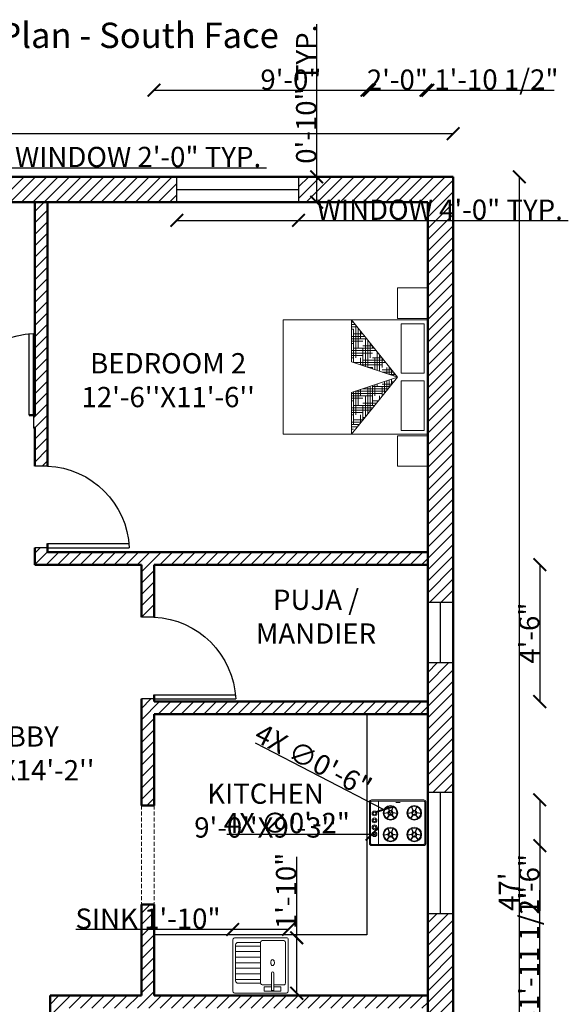
# Model space of a CAD drawing. Units: inches. Extents: x 1875 to 2385, y 1585 to 2263.
# Tile 3 of 3: x 2168 to 2385, y 1875 to 2263. Entities that reach past the tile are written whole.
import ezdxf

# ---------------------------------------------------------------- set-up
doc = ezdxf.new("R2010")
doc.units = ezdxf.units.IN
doc.header["$LTSCALE"] = 0.5
doc.linetypes.add('HIDDEN', pattern=[9.525, 6.35, -3.175])
for name, color, linetype, lineweight in [('A-ANNO-DIMS', 2, 'Continuous', 18), ('A-ANNO-TEXT', 7, 'Continuous', 25), ('A-AREA-IDEN', 7, 'Continuous', 25), ('A-EQPM', 9, 'Continuous', 18), ('A-FLOR-FIXT', 9, 'Continuous', 18), ('A-FURN', 8, 'Continuous', 18), ('A-WALL-HIDN', 56, 'HIDDEN', 18), ('A-WALL-PATT', 8, 'Continuous', 13), ('Doors', 42, 'Continuous', 25), ('kitchen', 70, 'Continuous', 25), ('Walls', 7, 'Continuous', 50), ('Windows', 140, 'Continuous', 25)]:
    doc.layers.add(name, color=color, linetype=linetype, lineweight=lineweight)
doc.styles.get("Standard").update_dxf_attribs({"font": 'arial.ttf'})
doc.dimstyles.get("Standard").update_dxf_attribs({"dimtxt": 8, "dimasz": 5, "dimexe": 0.18, "dimexo": 0.0625, "dimgap": 0.09, "dimtad": 1, "dimdec": 1, "dimzin": 0, "dimdsep": 46, "dimlunit": 4, "dimtxsty": 'Standard', "dimblk": 'ARCHTICK', "dimcen": 0.09, "dimse1": 1, "dimse2": 1, "dimadec": 0, "dimazin": 0, "dimtfac": 1, "dimtdec": 1, "dimtofl": 0, "dimtmove": 0, "dimatfit": 3, "dimfxl": 1, "dimtolj": 1, "dimtzin": 0, "dimarcsym": 0})

# ---------------------------------------------------------------- blocks, each defined once
blk = doc.blocks.new('AP0B05')
for p, q in [((35, 100), (35, 880)), ((75, 100), (75, 878.9)), ((35, 100), (35, -20)), ((815, 100), (815, -20))]:
    blk.add_line(p, q)
blk.add_lwpolyline([(35, 100), (75, 100)])
blk.add_arc((-2.4, 62.6), 818.3, 2.62122, 87.37878)
blk = doc.blocks.new('*X4')
at = {"color": 0}
for p, q in [((20.174, 14.75), (20.277, 14.75)), ((20.188, 14.75), (20.188, 14.767)), ((20.199, 14.781), (20.277, 14.781)), ((20.25, 14.812), (20.277, 14.812)), ((20.25, 14.319), (20.25, 14.75)), ((20.062, 14.257), (20.062, 14.612)), ((20.094, 14.375), (20.094, 14.65)), ((20.098, 14.656), (20.125, 14.656)), ((20.124, 14.688), (20.25, 14.688)), ((20.125, 14.5), (20.125, 14.689)), ((20.149, 14.719), (20.277, 14.719)), ((20.156, 14.625), (20.156, 14.728)), ((20.219, 14.309), (20.219, 14.625)), ((20.25, 14.625), (20.277, 14.625)), ((19.973, 14.5), (20.25, 14.5)), ((19.998, 14.531), (20.277, 14.531)), ((20, 14.237), (20, 14.5)), ((20.023, 14.562), (20.277, 14.562)), ((20.031, 14.247), (20.031, 14.573)), ((20.125, 14.594), (20.277, 14.594)), ((20.188, 14.299), (20.188, 14.5)), ((19.875, 14.25), (19.875, 14.379)), ((19.875, 14.344), (20.277, 14.344)), ((19.906, 14.375), (19.906, 14.417)), ((19.922, 14.438), (20, 14.438)), ((19.948, 14.469), (20.125, 14.469)), ((19.969, 14.226), (19.969, 14.375)), ((20, 14.375), (20.277, 14.375)), ((20.125, 14.406), (20.277, 14.406)), ((20.156, 14.288), (20.156, 14.375)), ((20.25, 14.438), (20.277, 14.438)), ((19.746, 14.219), (19.875, 14.219)), ((19.75, 14.154), (19.75, 14.223)), ((19.772, 14.25), (20, 14.25)), ((19.781, 14.164), (19.781, 14.262)), ((19.797, 14.281), (20.125, 14.281)), ((19.812, 14.174), (19.812, 14.301)), ((19.822, 14.312), (20.229, 14.312)), ((19.844, 14.185), (19.844, 14.34)), ((19.938, 14.216), (19.938, 14.25)), ((19.702, 14.094), (19.779, 14.094)), ((19.719, 14.073), (19.719, 14.114)), ((19.721, 14.188), (19.75, 14.188)), ((19.75, 14.034), (19.75, 14.103)), ((19.781, 13.995), (19.781, 14.093)), ((19.727, 14.062), (19.873, 14.062)), ((19.752, 14.031), (19.875, 14.031)), ((19.812, 14), (19.812, 14.082)), ((19.875, 13.878), (19.875, 14)), ((19.875, 13.969), (20.156, 13.969)), ((19.906, 13.84), (19.906, 14.051)), ((19.938, 13.801), (19.938, 14.041)), ((19.969, 13.875), (19.969, 14.031)), ((20, 14), (20, 14.02)), ((20, 14), (20.061, 14)), ((20.062, 13.645), (20.062, 14)), ((20.094, 13.625), (20.094, 13.989)), ((20.125, 13.75), (20.125, 13.979)), ((20.156, 13.875), (20.156, 13.969)), ((19.827, 13.938), (20.25, 13.938)), ((19.853, 13.906), (20.125, 13.906)), ((19.878, 13.875), (20, 13.875)), ((20.031, 13.684), (20.031, 13.875)), ((20.125, 13.844), (20.277, 13.844)), ((20.219, 13.451), (20.219, 13.875)), ((20.25, 13.5), (20.25, 13.937)), ((20.25, 13.875), (20.277, 13.875)), ((19.953, 13.781), (20.277, 13.781)), ((19.978, 13.75), (20.25, 13.75)), ((20, 13.812), (20.277, 13.812)), ((20, 13.723), (20, 13.75)), ((20.003, 13.719), (20.125, 13.719)), ((20.188, 13.49), (20.188, 13.75)), ((20.079, 13.625), (20.277, 13.625)), ((20.104, 13.594), (20.277, 13.594)), ((20.125, 13.656), (20.277, 13.656)), ((20.156, 13.529), (20.156, 13.625)), ((20.25, 13.688), (20.277, 13.688)), ((20.129, 13.562), (20.25, 13.562)), ((20.205, 13.469), (20.277, 13.469)), ((20.25, 13.5), (20.277, 13.5)), ((20.23, 13.438), (20.277, 13.438)), ((20.255, 13.406), (20.277, 13.406))]:
    blk.add_line(p, q, dxfattribs=at)
blk = doc.blocks.new('MAT-P13')
for p, q in [((-1.17, 0), (-1.17, -0.4)), ((-1.17, 0), (-0.77, 0)), ((-0.77, 0), (-0.77, -0.4)), ((-0.75, 0), (0.75, 0)), ((-0.75, 0), (-0.75, -1.9)), ((0.75, 0), (0.75, -1.9)), ((0.77, 0), (1.17, 0)), ((0.77, 0), (0.77, -0.4)), ((1.17, 0), (1.17, -0.4)), ((-0.7, -0.05), (-0.7, -0.35)), ((-0.7, -0.05), (-0.05, -0.05)), ((-0.05, -0.35), (-0.05, -0.05)), ((0.05, -0.05), (0.7, -0.05)), ((0.05, -0.35), (0.05, -0.05)), ((0.7, -0.05), (0.7, -0.35)), ((-0.7, -0.35), (-0.05, -0.35)), ((0.05, -0.35), (0.7, -0.35)), ((-1.17, -0.4), (-0.77, -0.4)), ((-0.75, -1.003), (0, -0.4)), ((0, -0.4), (-0.75, -1.003)), ((0, -0.4), (-0.2, -1.003)), ((0, -0.4), (0.2, -1.003)), ((0, -0.4), (0.75, -1.003)), ((0.77, -0.4), (1.17, -0.4)), ((-0.75, -1.003), (-0.2, -1.003)), ((0.2, -1.003), (0.75, -1.003)), ((0.75, -1.9), (-0.75, -1.9))]:
    blk.add_line(p, q)
at = {"xscale": -1, "rotation": 90}
blk.add_blockref('*X4', (14.128, 19.274), dxfattribs=at)
blk = doc.blocks.new('S_SINK12')
for p, q in [((0.25, 0.45), (0.25, 0)), ((0.35, 0.45), (0.35, 0)), ((0.45, 0.45), (0.45, 0)), ((0.55, 0.45), (0.55, 0)), ((0.65, 0.45), (0.65, 0)), ((0.75, 0.45), (0.75, 0)), ((0.85, 0.45), (0.85, 0))]:
    blk.add_line(p, q)
for points in [[(0, -0.469), (0, 0.469, -0.310961), (0.05, 0.5), (0.95, 0.5, -0.310466), (1, 0.469), (1, -0.469, -0.414214), (0.969, -0.5), (0.05, -0.5, -0.309971)], [(0.052, -0.195), (0.052, -0.242), (0.362, -0.242, 1), (0.362, -0.195)], [(0.5, -0.217), (0.503, -0.229, 0.107136), (0.516, -0.241, 0.076468), (0.534, -0.249), (0.554, -0.251), (0.575, -0.248, 0.076468), (0.592, -0.241, 0.107136), (0.604, -0.229), (0.608, -0.217), (0.604, -0.205, 0.107136), (0.592, -0.193, 0.076468), (0.575, -0.186), (0.554, -0.183), (0.532, -0.186, 0.076468), (0.516, -0.193, 0.107136), (0.503, -0.205)]]:
    blk.add_lwpolyline(points, format="xyb", close=True)
for points in [[(0.185, -0.001), (0.185, 0.419, -0.310466), (0.235, 0.45), (0.862, 0.45, -0.310466), (0.912, 0.419), (0.912, 0, -0.310466)], [(0.15, -0.195), (0.15, -0.031, -0.310466), (0.2, 0), (0.9, 0, -0.310466), (0.95, -0.031), (0.95, -0.419, -0.310466), (0.9, -0.45), (0.2, -0.45), (0.18, -0.448, -0.071009), (0.165, -0.442, -0.106323), (0.153, -0.432), (0.15, -0.422), (0.151, -0.419)]]:
    blk.add_lwpolyline(points, format="xyb")
for points in [[(0.114, -0.242), (0.114, -0.364), (0.039, -0.364), (0.039, -0.064), (0.114, -0.064), (0.114, -0.195)], [(0.15, -0.419), (0.15, -0.242)]]:
    blk.add_lwpolyline(points)
blk = doc.blocks.new('_ArchTick')
at = {"color": 0, "linetype": 'ByBlock', "const_width": 0.15}
blk.add_lwpolyline([(-0.5, -0.5), (0.5, 0.5)], dxfattribs=at)
blk = doc.blocks.new('*D12')
at = {"layer": 'A-ANNO-DIMS', "color": 0, "lineweight": -2, "ltscale": 0.5, "transparency": 16777216}
blk.add_line((1943.28, 2218.51), (2339.28, 2218.51), dxfattribs=at)
at = {"layer": 'Defpoints', "color": 0, "ltscale": 0.5, "transparency": 16777216}
for p in [(2339.28, 2218.51), (1943.28, 2201.46), (2339.28, 2201.46)]:
    blk.add_point(p, dxfattribs=at)
at = {"layer": 'A-ANNO-DIMS', "color": 0, "lineweight": -2, "ltscale": 0.5, "transparency": 16777216, "xscale": 5, "yscale": 5, "zscale": 5, "rotation": 180}
blk.add_blockref('_ArchTick', (1943.28, 2218.51), dxfattribs=at)
at = {"layer": 'A-ANNO-DIMS', "color": 0, "lineweight": -2, "ltscale": 0.5, "transparency": 16777216, "xscale": 5, "yscale": 5, "zscale": 5}
blk.add_blockref('_ArchTick', (2339.28, 2218.51), dxfattribs=at)
at = {"layer": 'A-ANNO-DIMS', "color": 0, "ltscale": 0.5, "transparency": 16777216, "insert": (2141.28, 2222.69), "char_height": 8, "attachment_point": 5}
blk.add_mtext("\\A1;33'", dxfattribs=at)
blk = doc.blocks.new('*D13')
at = {"layer": 'A-ANNO-DIMS', "color": 0, "lineweight": -2, "ltscale": 0.5, "transparency": 16777216}
blk.add_line((2365.35, 2201.46), (2365.35, 1637.46), dxfattribs=at)
at = {"layer": 'Defpoints', "color": 0, "ltscale": 0.5, "transparency": 16777216}
for p in [(2339.28, 2201.46), (2339.28, 1637.46), (2365.35, 1637.46)]:
    blk.add_point(p, dxfattribs=at)
at = {"layer": 'A-ANNO-DIMS', "color": 0, "lineweight": -2, "ltscale": 0.5, "transparency": 16777216, "xscale": 5, "yscale": 5, "zscale": 5}
for p, rotation in [((2365.35, 2201.46), 90), ((2365.35, 1637.46), 270)]:
    blk.add_blockref('_ArchTick', p, dxfattribs=dict(at, rotation=rotation))
at = {"layer": 'A-ANNO-DIMS', "color": 0, "ltscale": 0.5, "transparency": 16777216, "insert": (2361.26, 1919.46), "char_height": 8, "attachment_point": 5, "rotation": 90}
blk.add_mtext("\\A1;47'", dxfattribs=at)
blk = doc.blocks.new('WIN-48IN')
at = {"ltscale": 0.5}
blk.add_line((0, 0), (48, 0), dxfattribs=at)
blk.add_lwpolyline([(0, 5), (48, 5), (48, -5), (0, -5)], close=True, dxfattribs=at)
blk = doc.blocks.new('WIN-24IN')
at = {"ltscale": 0.5}
blk.add_line((0, 0), (24, 0), dxfattribs=at)
blk.add_lwpolyline([(0, 5), (24, 5), (24, -5), (0, -5)], close=True, dxfattribs=at)
blk = doc.blocks.new('COOKTOP-BURNER')
for points in [[(-2.56, -0.11), (-0.95, 0.12, 0.472071), (-0.53, 0.81), (-1.08, 2.32)], [(-2.55, -0.29), (-0.93, -0.05, 0.472479), (-0.37, 0.87), (-0.92, 2.39)], [(2.55, -0.26), (0.93, -0.05, -0.472479), (0.36, 0.87), (0.9, 2.4)], [(2.56, -0.09), (0.95, 0.12, -0.472071), (0.52, 0.81), (1.06, 2.33)], [(1.66, -1.95), (0.56, -0.74, 0.472479), (-0.51, -0.79), (-1.47, -2.1)], [(1.52, -2.06), (0.44, -0.86, 0.472071), (-0.37, -0.89), (-1.33, -2.19)]]:
    blk.add_lwpolyline(points, format="xyb")
for radius in [2.9, 2.56]:
    blk.add_circle((0, 0), radius)
for radius, start, end in [(0.99, 123.0309, 173.5763), (0.82, 127.8377, 168.7328), (0.99, 67.462, 113.0371), (0.82, 65.9407, 114.5584), (0.82, 11.7663, 52.6614), (0.99, 6.9228, 57.4682), (0.99, 183.6067, 236.9387), (0.82, 182.012, 238.4601), (0.99, 246.9326, 297.478), (0.82, 251.7394, 292.6344), (0.82, 305.9137, 358.4871), (0.99, 307.5084, 356.8924)]:
    blk.add_arc((0, 0), radius, start, end)
blk = doc.blocks.new('COOKTOP-CONTROL')
for radius in [0.939, 0.534]:
    blk.add_circle((0, 0), radius)
blk = doc.blocks.new('*D22')
at = {"layer": 'A-ANNO-DIMS', "color": 0, "lineweight": -2, "ltscale": 0.5, "transparency": 16777216}
for p, q in [((2230.28, 2184.26), (2278.28, 2184.26)), ((2278.28, 2184.26), (2384.7, 2184.26))]:
    blk.add_line(p, q, dxfattribs=at)
at = {"layer": 'Defpoints', "color": 0, "ltscale": 0.5, "transparency": 16777216}
for p in [(2230.28, 2191.46), (2278.28, 2191.46), (2278.28, 2184.26)]:
    blk.add_point(p, dxfattribs=at)
at = {"layer": 'A-ANNO-DIMS', "color": 0, "lineweight": -2, "ltscale": 0.5, "transparency": 16777216, "xscale": 5, "yscale": 5, "zscale": 5, "rotation": 180}
blk.add_blockref('_ArchTick', (2230.28, 2184.26), dxfattribs=at)
at = {"layer": 'A-ANNO-DIMS', "color": 0, "lineweight": -2, "ltscale": 0.5, "transparency": 16777216, "xscale": 5, "yscale": 5, "zscale": 5}
blk.add_blockref('_ArchTick', (2278.28, 2184.26), dxfattribs=at)
at = {"layer": 'A-ANNO-DIMS', "color": 0, "ltscale": 0.5, "transparency": 16777216, "insert": (2333.99, 2188.49), "char_height": 8, "attachment_point": 5}
blk.add_mtext('\\A1;WINDOW 4\'-0" TYP.', dxfattribs=at)
blk = doc.blocks.new('*D23')
at = {"layer": 'A-ANNO-DIMS', "color": 0, "lineweight": -2, "ltscale": 0.5, "transparency": 16777216}
for p, q in [((2285.48, 2201.46), (2285.48, 2261.62)), ((2285.48, 2191.46), (2285.48, 2201.46))]:
    blk.add_line(p, q, dxfattribs=at)
at = {"layer": 'Defpoints', "color": 0, "ltscale": 0.5, "transparency": 16777216}
for p in [(2278.28, 2201.46), (2285.48, 2201.46), (2278.28, 2191.46)]:
    blk.add_point(p, dxfattribs=at)
at = {"layer": 'A-ANNO-DIMS', "color": 0, "lineweight": -2, "ltscale": 0.5, "transparency": 16777216, "xscale": 5, "yscale": 5, "zscale": 5}
for p, rotation in [((2285.48, 2201.46), 90), ((2285.48, 2191.46), 270)]:
    blk.add_blockref('_ArchTick', p, dxfattribs=dict(at, rotation=rotation))
at = {"layer": 'A-ANNO-DIMS', "color": 0, "ltscale": 0.5, "transparency": 16777216, "insert": (2281.31, 2234.04), "char_height": 8, "attachment_point": 5, "rotation": 90}
blk.add_mtext('\\A1;0\'-10" TYP.', dxfattribs=at)
blk = doc.blocks.new('*D26')
at = {"layer": 'A-ANNO-DIMS', "color": 0, "lineweight": -2, "ltscale": 0.5, "transparency": 16777216}
for p, q in [((2135.28, 2205.06), (2159.28, 2205.06)), ((2159.28, 2205.06), (2265.7, 2205.06))]:
    blk.add_line(p, q, dxfattribs=at)
at = {"layer": 'Defpoints', "color": 0, "ltscale": 0.5, "transparency": 16777216}
for p in [(2159.28, 2205.06), (2135.28, 2201.46), (2159.28, 2201.46)]:
    blk.add_point(p, dxfattribs=at)
at = {"layer": 'A-ANNO-DIMS', "color": 0, "lineweight": -2, "ltscale": 0.5, "transparency": 16777216, "xscale": 5, "yscale": 5, "zscale": 5, "rotation": 180}
blk.add_blockref('_ArchTick', (2135.28, 2205.06), dxfattribs=at)
at = {"layer": 'A-ANNO-DIMS', "color": 0, "lineweight": -2, "ltscale": 0.5, "transparency": 16777216, "xscale": 5, "yscale": 5, "zscale": 5}
blk.add_blockref('_ArchTick', (2159.28, 2205.06), dxfattribs=at)
at = {"layer": 'A-ANNO-DIMS', "color": 0, "ltscale": 0.5, "transparency": 16777216, "insert": (2214.99, 2209.29), "char_height": 8, "attachment_point": 5}
blk.add_mtext('\\A1;WINDOW 2\'-0" TYP.', dxfattribs=at)
blk = doc.blocks.new('*D34')
at = {"layer": 'A-ANNO-DIMS', "color": 0, "lineweight": -2, "ltscale": 0.5, "transparency": 16777216}
for p, q in [((2252.3, 1904.61), (2190.49, 1904.61)), ((2274.27, 1904.61), (2252.3, 1904.61))]:
    blk.add_line(p, q, dxfattribs=at)
at = {"layer": 'Defpoints', "color": 0, "ltscale": 0.5, "transparency": 16777216}
for p in [(2252.3, 1904.61), (2252.3, 1901.31), (2274.27, 1901.31)]:
    blk.add_point(p, dxfattribs=at)
at = {"layer": 'A-ANNO-DIMS', "color": 0, "lineweight": -2, "ltscale": 0.5, "transparency": 16777216, "xscale": 5, "yscale": 5, "zscale": 5, "rotation": 180}
blk.add_blockref('_ArchTick', (2252.3, 1904.61), dxfattribs=at)
at = {"layer": 'A-ANNO-DIMS', "color": 0, "lineweight": -2, "ltscale": 0.5, "transparency": 16777216, "xscale": 5, "yscale": 5, "zscale": 5}
blk.add_blockref('_ArchTick', (2274.27, 1904.61), dxfattribs=at)
at = {"layer": 'A-ANNO-DIMS', "color": 0, "ltscale": 0.5, "transparency": 16777216, "insert": (2218.9, 1908.83), "char_height": 8, "attachment_point": 5}
blk.add_mtext('\\A1;SINK 1\'-10"', dxfattribs=at)
blk = doc.blocks.new('*D35')
at = {"layer": 'A-ANNO-DIMS', "color": 0, "lineweight": -2, "ltscale": 0.5, "transparency": 16777216}
for p, q in [((2277.56, 1901.31), (2277.56, 1933.22)), ((2277.56, 1879.39), (2277.56, 1901.31))]:
    blk.add_line(p, q, dxfattribs=at)
at = {"layer": 'Defpoints', "color": 0, "ltscale": 0.5, "transparency": 16777216}
for p in [(2274.27, 1901.31), (2277.56, 1901.31), (2274.27, 1879.39)]:
    blk.add_point(p, dxfattribs=at)
at = {"layer": 'A-ANNO-DIMS', "color": 0, "lineweight": -2, "ltscale": 0.5, "transparency": 16777216, "xscale": 5, "yscale": 5, "zscale": 5}
for p, rotation in [((2277.56, 1901.31), 90), ((2277.56, 1879.39), 270)]:
    blk.add_blockref('_ArchTick', p, dxfattribs=dict(at, rotation=rotation))
at = {"layer": 'A-ANNO-DIMS', "color": 0, "ltscale": 0.5, "transparency": 16777216, "insert": (2273.39, 1919.77), "char_height": 8, "attachment_point": 5, "rotation": 90}
blk.add_mtext('\\A1;1\'-10"', dxfattribs=at)
blk = doc.blocks.new('*D38')
at = {"layer": 'A-ANNO-DIMS', "color": 0, "lineweight": -2, "ltscale": 0.5, "transparency": 16777216}
blk.add_line((2373.43, 2048.46), (2373.43, 1994.46), dxfattribs=at)
at = {"layer": 'Defpoints', "color": 0, "ltscale": 0.5, "transparency": 16777216}
for p in [(2329.28, 2048.46), (2329.28, 1994.46), (2373.43, 1994.46)]:
    blk.add_point(p, dxfattribs=at)
at = {"layer": 'A-ANNO-DIMS', "color": 0, "lineweight": -2, "ltscale": 0.5, "transparency": 16777216, "xscale": 5, "yscale": 5, "zscale": 5}
for p, rotation in [((2373.43, 2048.46), 90), ((2373.43, 1994.46), 270)]:
    blk.add_blockref('_ArchTick', p, dxfattribs=dict(at, rotation=rotation))
at = {"layer": 'A-ANNO-DIMS', "color": 0, "ltscale": 0.5, "transparency": 16777216, "insert": (2369.26, 2021.46), "char_height": 8, "attachment_point": 5, "rotation": 90}
blk.add_mtext('\\A1;4\'-6"', dxfattribs=at)
blk = doc.blocks.new('*D39')
at = {"layer": 'A-ANNO-DIMS', "color": 0, "lineweight": -2, "ltscale": 0.5, "transparency": 16777216}
blk.add_line((2221.28, 2235.61), (2329.28, 2235.61), dxfattribs=at)
at = {"layer": 'Defpoints', "color": 0, "ltscale": 0.5, "transparency": 16777216}
for p in [(2329.28, 2235.61), (2221.28, 2048.46), (2329.28, 2048.46)]:
    blk.add_point(p, dxfattribs=at)
at = {"layer": 'A-ANNO-DIMS', "color": 0, "lineweight": -2, "ltscale": 0.5, "transparency": 16777216, "xscale": 5, "yscale": 5, "zscale": 5, "rotation": 180}
blk.add_blockref('_ArchTick', (2221.28, 2235.61), dxfattribs=at)
at = {"layer": 'A-ANNO-DIMS', "color": 0, "lineweight": -2, "ltscale": 0.5, "transparency": 16777216, "xscale": 5, "yscale": 5, "zscale": 5}
blk.add_blockref('_ArchTick', (2329.28, 2235.61), dxfattribs=at)
at = {"layer": 'A-ANNO-DIMS', "color": 0, "ltscale": 0.5, "transparency": 16777216, "insert": (2275.28, 2239.78), "char_height": 8, "attachment_point": 5}
blk.add_mtext('\\A1;9\'-0"', dxfattribs=at)
blk = doc.blocks.new('*D44')
at = {"layer": 'A-ANNO-DIMS', "color": 0, "lineweight": -2, "ltscale": 0.5, "transparency": 16777216}
blk.add_line((2305.28, 2235.61), (2329.28, 2235.61), dxfattribs=at)
at = {"layer": 'Defpoints', "color": 0, "ltscale": 0.5, "transparency": 16777216}
for p in [(2329.28, 2235.61), (2305.28, 1989.46), (2329.28, 1989.46)]:
    blk.add_point(p, dxfattribs=at)
at = {"layer": 'A-ANNO-DIMS', "color": 0, "lineweight": -2, "ltscale": 0.5, "transparency": 16777216, "xscale": 5, "yscale": 5, "zscale": 5, "rotation": 180}
blk.add_blockref('_ArchTick', (2305.28, 2235.61), dxfattribs=at)
at = {"layer": 'A-ANNO-DIMS', "color": 0, "lineweight": -2, "ltscale": 0.5, "transparency": 16777216, "xscale": 5, "yscale": 5, "zscale": 5}
blk.add_blockref('_ArchTick', (2329.28, 2235.61), dxfattribs=at)
at = {"layer": 'A-ANNO-DIMS', "color": 0, "ltscale": 0.5, "transparency": 16777216, "insert": (2317.28, 2239.78), "char_height": 8, "attachment_point": 5}
blk.add_mtext('\\A1;2\'-0"', dxfattribs=at)
blk = doc.blocks.new('*D45')
at = {"layer": 'A-ANNO-DIMS', "color": 0, "lineweight": -2, "ltscale": 0.5, "transparency": 16777216}
for p, q in [((2306.22, 2235.61), (2328.55, 2235.61)), ((2328.55, 2235.61), (2379.1, 2235.61))]:
    blk.add_line(p, q, dxfattribs=at)
at = {"layer": 'Defpoints', "color": 0, "ltscale": 0.5, "transparency": 16777216}
for p in [(2328.55, 2235.61), (2306.22, 1954.82), (2328.55, 1954.82)]:
    blk.add_point(p, dxfattribs=at)
at = {"layer": 'A-ANNO-DIMS', "color": 0, "lineweight": -2, "ltscale": 0.5, "transparency": 16777216, "xscale": 5, "yscale": 5, "zscale": 5, "rotation": 180}
blk.add_blockref('_ArchTick', (2306.22, 2235.61), dxfattribs=at)
at = {"layer": 'A-ANNO-DIMS', "color": 0, "lineweight": -2, "ltscale": 0.5, "transparency": 16777216, "xscale": 5, "yscale": 5, "zscale": 5}
blk.add_blockref('_ArchTick', (2328.55, 2235.61), dxfattribs=at)
at = {"layer": 'A-ANNO-DIMS', "color": 0, "ltscale": 0.5, "transparency": 16777216, "insert": (2356.33, 2239.84), "char_height": 8, "attachment_point": 5}
blk.add_mtext('\\A1;1\'-10 1/2"', dxfattribs=at)
blk = doc.blocks.new('*D46')
at = {"layer": 'A-ANNO-DIMS', "color": 0, "lineweight": -2, "ltscale": 0.5, "transparency": 16777216}
for p, q in [((2373.43, 1955.68), (2373.43, 1937.65)), ((2373.43, 1937.65), (2373.43, 1911.96))]:
    blk.add_line(p, q, dxfattribs=at)
at = {"layer": 'Defpoints', "color": 0, "ltscale": 0.5, "transparency": 16777216}
for p in [(2327.7, 1955.68), (2327.7, 1937.65), (2373.43, 1937.65)]:
    blk.add_point(p, dxfattribs=at)
at = {"layer": 'A-ANNO-DIMS', "color": 0, "lineweight": -2, "ltscale": 0.5, "transparency": 16777216, "xscale": 5, "yscale": 5, "zscale": 5}
for p, rotation in [((2373.43, 1955.68), 90), ((2373.43, 1937.65), 270)]:
    blk.add_blockref('_ArchTick', p, dxfattribs=dict(at, rotation=rotation))
at = {"layer": 'A-ANNO-DIMS', "color": 0, "ltscale": 0.5, "transparency": 16777216, "insert": (2369.26, 1922.3), "char_height": 8, "attachment_point": 5, "rotation": 90}
blk.add_mtext('\\A1;1\'-6"', dxfattribs=at)
blk = doc.blocks.new('*D48')
at = {"layer": 'A-ANNO-DIMS', "color": 0, "lineweight": -2, "ltscale": 0.5, "transparency": 16777216}
for p, q in [((2373.43, 1869.47), (2373.43, 1920.02)), ((2373.43, 1846.07), (2373.43, 1869.47))]:
    blk.add_line(p, q, dxfattribs=at)
at = {"layer": 'Defpoints', "color": 0, "ltscale": 0.5, "transparency": 16777216}
for p in [(2326.3, 1869.47), (2373.43, 1869.47), (2326.3, 1846.07)]:
    blk.add_point(p, dxfattribs=at)
at = {"layer": 'A-ANNO-DIMS', "color": 0, "lineweight": -2, "ltscale": 0.5, "transparency": 16777216, "xscale": 5, "yscale": 5, "zscale": 5}
for p, rotation in [((2373.43, 1869.47), 90), ((2373.43, 1846.07), 270)]:
    blk.add_blockref('_ArchTick', p, dxfattribs=dict(at, rotation=rotation))
at = {"layer": 'A-ANNO-DIMS', "color": 0, "ltscale": 0.5, "transparency": 16777216, "insert": (2369.21, 1897.24), "char_height": 8, "attachment_point": 5, "rotation": 90}
blk.add_mtext('\\A1;1\'-11 1/2"', dxfattribs=at)
blk = doc.blocks.new('*D49')
at = {"layer": 'A-ANNO-DIMS', "color": 0, "lineweight": -2, "ltscale": 0.5, "transparency": 16777216}
for p, q in [((2261.15, 1978.22), (2311.98, 1951.89)), ((2314.46, 1950.56), (2314.64, 1950.56)), ((2314.55, 1950.47), (2314.55, 1950.65))]:
    blk.add_line(p, q, dxfattribs=at)
at = {"layer": 'Defpoints', "color": 0, "ltscale": 0.5, "transparency": 16777216}
for p in [(2311.98, 1951.89), (2317.13, 1949.22)]:
    blk.add_point(p, dxfattribs=at)
at = {"layer": 'A-ANNO-DIMS', "color": 0, "lineweight": -2, "ltscale": 0.5, "transparency": 16777216, "xscale": 5, "yscale": 5, "zscale": 5, "rotation": 332.6167494791556}
blk.add_blockref('_ArchTick', (2311.98, 1951.89), dxfattribs=at)
at = {"layer": 'A-ANNO-DIMS', "color": 0, "ltscale": 0.5, "transparency": 16777216, "insert": (2284.15, 1971.26), "char_height": 8, "attachment_point": 5, "rotation": 332.6167}
blk.add_mtext('\\A1;4X ∅0\'-6"', dxfattribs=at)
blk = doc.blocks.new('*D50')
at = {"layer": 'A-ANNO-DIMS', "color": 0, "lineweight": -2, "ltscale": 0.5, "transparency": 16777216}
for p, q in [((2250.06, 1942.18), (2307.3, 1942.14)), ((2308.15, 1942.14), (2308.33, 1942.14)), ((2308.24, 1942.05), (2308.24, 1942.23))]:
    blk.add_line(p, q, dxfattribs=at)
at = {"layer": 'Defpoints', "color": 0, "ltscale": 0.5, "transparency": 16777216}
for p in [(2307.3, 1942.14), (2309.18, 1942.14)]:
    blk.add_point(p, dxfattribs=at)
at = {"layer": 'A-ANNO-DIMS', "color": 0, "lineweight": -2, "ltscale": 0.5, "transparency": 16777216, "xscale": 5, "yscale": 5, "zscale": 5, "rotation": 359.9647327650331}
blk.add_blockref('_ArchTick', (2307.3, 1942.14), dxfattribs=at)
at = {"layer": 'A-ANNO-DIMS', "color": 0, "ltscale": 0.5, "transparency": 16777216, "insert": (2273.68, 1946.56), "char_height": 8, "attachment_point": 5, "rotation": 359.9647}
blk.add_mtext('\\A1;4X ∅0\'-2"', dxfattribs=at)

msp = doc.modelspace()

# ---------------------------------------------------------------- hatches: boundary and pattern name
at = {"layer": 'A-WALL-PATT', "ltscale": 0.5, "transparency": 33554585}
h = msp.add_hatch(dxfattribs=at)
h.set_pattern_fill('ANSI31', color=256)
h.paths.add_polyline_path([(2010.28, 2201.46), (1943.28, 2201.46), (1943.28, 1986.92), (1953.28, 1986.92), (1953.28, 2191.46), (2010.28, 2191.46)])
h.paths.add_polyline_path([(2135.28, 2201.46), (2058.28, 2201.46), (2058.28, 2191.46), (2135.28, 2191.46)])
h.paths.add_polyline_path([(2120.28, 2191.46), (2115.28, 2191.46), (2115.28, 2087.38), (2120.28, 2087.38), (2120.28, 2102.46), (2141.45, 2102.46), (2141.45, 2107.46), (2120.28, 2107.46)])
h.paths.add_polyline_path([(2230.28, 2201.46), (2159.28, 2201.46), (2159.28, 2191.46), (2160.9, 2191.46), (2230.28, 2191.46)])
h.paths.add_polyline_path([(2179.28, 2191.46), (2174.28, 2191.46), (2174.28, 2107.46), (2173.71, 2107.46), (2173.71, 2107.42), (2173.71, 2102.46), (2174.28, 2102.46), (2174.28, 2087.38), (2179.28, 2087.38)])
h.paths.add_polyline_path([(2339.28, 2201.46), (2278.28, 2201.46), (2278.28, 2191.46), (2329.28, 2191.46), (2329.28, 2033.69), (2339.28, 2033.69)])
h.paths.add_polyline_path([(2329.28, 2053.46), (2179.28, 2053.46), (2179.28, 2055.12), (2179.25, 2055.12), (2174.28, 2055.12), (2174.28, 2048.46), (2216.28, 2048.46), (2216.28, 2027.77), (2221.28, 2027.77), (2221.28, 2048.46), (2329.28, 2048.46)])
h = msp.add_hatch(dxfattribs=at)
h.set_pattern_fill('ANSI31', color=256)
h.paths.add_polyline_path([(2120.28, 2055.12), (2115.28, 2055.12), (2115.28, 2053.46), (1953.28, 2053.46), (1953.28, 2048.46), (2120.28, 2048.46)])
h.paths.add_polyline_path([(2339.28, 2009.69), (2329.28, 2009.69), (2329.28, 1958.74), (2339.28, 1958.74)])
h.paths.add_polyline_path([(2140.01, 1729.46), (2138.58, 1729.46), (2120.28, 1729.46), (2120.28, 1988.46), (2115.28, 1988.46), (2115.28, 1878.46), (2106.32, 1878.46), (2106.32, 1878.42), (2106.32, 1873.46), (2110.28, 1873.46), (2110.28, 1719.46), (2140.01, 1719.46)])
h.paths.add_polyline_path([(2074.06, 1878.46), (1953.28, 1878.46), (1953.28, 1873.46), (2074.06, 1873.46)])
h.paths.add_polyline_path([(1953.28, 1938.92), (1943.28, 1938.92), (1943.28, 1637.46), (1953.28, 1637.46), (1953.28, 1647.46)])
h.paths.add_polyline_path([(2329.28, 1729.46), (2164.01, 1729.46), (2164.01, 1719.46), (2329.28, 1719.46)])
h.paths.add_polyline_path([(2185.28, 1837.05), (2180.28, 1837.05), (2180.28, 1818.46), (2158.46, 1818.46), (2158.46, 1813.46), (2180.28, 1813.46), (2180.28, 1729.46), (2185.28, 1729.46)])
h.paths.add_polyline_path([(2126.2, 1818.46), (2120.28, 1818.46), (2120.28, 1813.46), (2126.2, 1813.46), (2126.2, 1813.5)], flags=17)
h.paths.add_polyline_path([(2339.28, 1910.74), (2329.28, 1910.74), (2329.28, 1823.21), (2339.28, 1823.21)])
h.paths.add_polyline_path([(2339.28, 1775.21), (2329.28, 1775.21), (2329.28, 1701.57), (2339.28, 1701.57)])
h.paths.add_polyline_path([(2339.28, 1665.57), (2329.28, 1665.57), (2329.28, 1647.46), (2110.28, 1647.46), (2102.69, 1647.46), (2102.69, 1637.46), (2110.28, 1637.46), (2339.28, 1637.46)])
h = msp.add_hatch(dxfattribs=at)
h.set_pattern_fill('ANSI31', color=256)
h.paths.add_polyline_path([(2329.28, 1994.46), (2221.28, 1994.46), (2221.28, 1995.51), (2221.25, 1995.51), (2216.28, 1995.51), (2216.28, 1953.46), (2221.28, 1953.46), (2221.28, 1989.46), (2329.28, 1989.46)])
h.paths.add_polyline_path([(2221.28, 1914.46), (2216.28, 1914.46), (2216.28, 1878.46), (2180.28, 1878.46), (2180.28, 1869.31), (2185.28, 1869.31), (2185.28, 1873.46), (2329.28, 1873.46), (2329.28, 1878.46), (2221.28, 1878.46)])

# ---------------------------------------------------------------- linework, layer by layer
at = {"layer": 'A-EQPM'}
msp.add_line((2309.77, 1955.2), (2309.77, 1938.13), dxfattribs=at)
for points in [[(2327.7, 1937.65), (2307.08, 1937.65, -0.414214), (2306.22, 1938.5), (2306.22, 1954.82, -0.414214), (2307.08, 1955.68), (2327.7, 1955.68, -0.414214), (2328.55, 1954.82), (2328.55, 1938.5, -0.414214)], [(2327.7, 1938.13), (2307.08, 1938.13, -0.414214), (2306.7, 1938.5), (2306.7, 1954.82, -0.414214), (2307.08, 1955.2), (2327.7, 1955.2, -0.414214), (2328.08, 1954.82), (2328.08, 1938.5, -0.414214)]]:
    msp.add_lwpolyline(points, format="xyb", close=True, dxfattribs=at)
msp.add_lwpolyline([(2316.6, 1954.65), (2318.31, 1954.65), (2318.31, 1954.59), (2316.6, 1954.59)], close=True, dxfattribs=at)
at = {"layer": 'A-WALL-HIDN', "ltscale": 0.5}
for p, q in [((2216.28, 1953.46), (2216.28, 1914.46)), ((2221.28, 1953.46), (2221.28, 1914.46))]:
    msp.add_line(p, q, dxfattribs=at)
at = {"layer": 'kitchen'}
msp.add_lwpolyline([(2305.28, 1989.46), (2305.28, 1902.46), (2221.28, 1902.46)], dxfattribs=at)
at = {"layer": 'Walls'}
for p, q in [((1943.28, 2201.46), (2339.28, 2201.46)), ((2339.28, 2201.46), (2339.28, 1637.46)), ((1953.28, 2191.46), (2329.28, 2191.46)), ((2174.28, 2191.46), (2174.28, 2107.46)), ((2179.28, 2191.46), (2179.28, 2087.38)), ((2329.28, 2191.46), (2329.28, 1647.46)), ((2172.05, 2107.46), (2174.28, 2107.46)), ((2173.71, 2102.46), (2174.28, 2102.46)), ((2174.28, 2102.46), (2174.28, 2087.38)), ((2174.28, 2055.12), (2174.28, 2048.46)), ((2179.28, 2056.77), (2179.28, 2053.46)), ((2179.28, 2053.46), (2329.28, 2053.46)), ((2174.28, 2048.46), (2216.28, 2048.46)), ((2216.28, 2048.46), (2216.28, 2027.77)), ((2221.28, 2048.46), (2221.28, 2027.76)), ((2221.28, 2048.46), (2329.28, 2048.46)), ((2221.28, 1997.16), (2221.28, 1994.46)), ((2216.28, 1995.51), (2216.28, 1987.27)), ((2216.28, 1995.51), (2216.28, 1953.46)), ((2221.28, 1994.46), (2329.28, 1994.46)), ((2221.28, 1989.46), (2329.28, 1989.46)), ((2221.28, 1989.46), (2221.28, 1985.62)), ((2221.28, 1989.46), (2221.28, 1953.46)), ((2216.28, 1914.46), (2216.28, 1878.46)), ((2221.28, 1914.46), (2221.28, 1878.46)), ((2180.28, 1878.46), (2216.28, 1878.46)), ((2180.28, 1878.46), (2180.28, 1869.31)), ((2180.28, 1878.46), (2180.28, 1869.31)), ((2221.28, 1878.46), (2329.28, 1878.46))]:
    msp.add_line(p, q, dxfattribs=at)
at = {"layer": 'Walls', "ltscale": 0.5}
for p, q in [((2221.28, 1953.46), (2216.28, 1953.46)), ((2221.28, 1914.46), (2216.28, 1914.46))]:
    msp.add_line(p, q, dxfattribs=at)

# ---------------------------------------------------------------- block references
at = {"layer": 'A-EQPM'}
for name, p in [('COOKTOP-CONTROL', (2308.24, 1950.33)), ('COOKTOP-BURNER', (2314.55, 1950.56)), ('COOKTOP-BURNER', (2323.92, 1950.56)), ('COOKTOP-CONTROL', (2308.24, 1947.6)), ('COOKTOP-CONTROL', (2308.24, 1944.87)), ('COOKTOP-CONTROL', (2308.24, 1942.14)), ('COOKTOP-BURNER', (2314.55, 1942.02)), ('COOKTOP-BURNER', (2323.92, 1942.02))]:
    msp.add_blockref(name, p, dxfattribs=at)
at = {"layer": 'A-FLOR-FIXT', "ltscale": 0.5, "xscale": 21.92158977240194, "yscale": 21.92158977240194, "zscale": 21.92158977240194, "rotation": 90}
msp.add_blockref('S_SINK12', (2263.28, 1879.39), dxfattribs=at)
at = {"layer": 'A-FURN', "ltscale": 0.5, "xscale": -30.05916968857566, "yscale": 30.05916968857566, "zscale": 30.05916968857566, "rotation": 270}
msp.add_blockref('MAT-P13', (2329.28, 2122.46), dxfattribs=at)
at = {"layer": 'Doors', "xscale": -0.0413587909994788, "yscale": 0.0413587909994788, "zscale": 0.0413587909994788}
msp.add_blockref('AP0B05', (2175.15, 2103.29), dxfattribs=at)
at = {"layer": 'Doors', "xscale": -0.0413587909994788, "yscale": 0.0413587909994788, "zscale": 0.0413587909994788, "rotation": 270}
for p in [(2175.11, 2053.67), (2217.11, 1994.06)]:
    msp.add_blockref('AP0B05', p, dxfattribs=at)
at = {"layer": 'Windows'}
msp.add_blockref('WIN-48IN', (2230.28, 2196.46), dxfattribs=at)
for name, p, rotation in [('WIN-24IN', (2334.28, 2009.69), 89.99999999999677), ('WIN-48IN', (2334.28, 1910.74), 89.9999999999985)]:
    msp.add_blockref(name, p, dxfattribs=dict(at, rotation=rotation))

# ---------------------------------------------------------------- texts
at = {"layer": 'A-ANNO-TEXT', "ltscale": 0.5}
msp.add_text('33X47 (1551 sq ft) House Plan - South Face', height=10, dxfattribs=at).set_placement((2002.52, 2252.29))
at = {"layer": 'A-AREA-IDEN', "ltscale": 0.5, "char_height": 8, "attachment_point": 1}
for s, insert in [("\\pxqc;BEDROOM 2\\P12'-6''X11'-6''", (2189.66, 2131.92)), ('\\pxqc;PUJA /\\PMANDIER', (2247.99, 2038.63)), ("\\pxqc;LOBBY\\P8'-0''X14'-2''", (2129.42, 1984.69)), ("\\pxqc;KITCHEN\\P9'-0''X9'-3''", (2228.07, 1962.14))]:
    msp.add_mtext_dynamic_manual_height_columns(s, width=74.3766, gutter_width=12.5, heights=[0], dxfattribs=dict(at, insert=insert))

# ---------------------------------------------------------------- dimensions: what is measured, and where the dimension line sits
at = {"layer": 'A-ANNO-DIMS', "ltscale": 0.5}
for base, p1, p2, angle, text, picture, middle in [((2285.48, 2201.46), (2278.28, 2191.46), (2278.28, 2201.46), 90, '<> TYP.', '*D23', (2281.31, 2234.04)), ((2252.3, 1904.61), (2274.27, 1901.31), (2252.3, 1901.31), 180, 'SINK <>', '*D34', (2218.9, 1908.83))]:
    dim = msp.add_linear_dim(base=base, p1=p1, p2=p2, angle=angle, text=text, dimstyle='Standard', override={"dimdec": 1, "dimlfac": 1, "dimrnd": 0, "dimzin": 1, "dimdsep": 46, "dimlunit": 4, "dimfrac": 2}, dxfattribs=at)
    dim.commit()
    dim.dimension.update_dxf_attribs({"geometry": picture, "text_midpoint": middle})
for base, p1, p2, override, picture, middle in [((2328.55, 2235.61), (2306.22, 1954.82), (2328.55, 1954.82), {"dimdec": 1, "dimlfac": 1, "dimrnd": 0, "dimzin": 1, "dimdsep": 46, "dimlunit": 4, "dimfrac": 2}, '*D45', (2356.33, 2239.84)), ((2329.28, 2235.61), (2221.28, 2048.46), (2329.28, 2048.46), {"dimdec": 1, "dimlfac": 1, "dimrnd": 0, "dimzin": 1, "dimdsep": 46, "dimlunit": 4, "dimfrac": 2}, '*D39', (2275.28, 2239.78)), ((2329.28, 2235.61), (2305.28, 1989.46), (2329.28, 1989.46), {"dimdec": 1, "dimlfac": 1, "dimrnd": 0, "dimzin": 1, "dimdsep": 46, "dimlunit": 4, "dimfrac": 2}, '*D44', (2317.28, 2239.78)), ((2339.28, 2218.51), (1943.28, 2201.46), (2339.28, 2201.46), {"dimclrd": 0, "dimclre": 0, "dimclrt": 0}, '*D12', (2141.28, 2222.69))]:
    dim = msp.add_linear_dim(base=base, p1=p1, p2=p2, dimstyle='Standard', override=override, dxfattribs=at)
    dim.commit()
    dim.dimension.update_dxf_attribs({"geometry": picture, "text_midpoint": middle})
for base, p1, p2, picture, middle in [((2159.28, 2205.06), (2135.28, 2201.46), (2159.28, 2201.46), '*D26', (2214.99, 2209.29)), ((2278.28, 2184.26), (2230.28, 2191.46), (2278.28, 2191.46), '*D22', (2333.99, 2188.49))]:
    dim = msp.add_linear_dim(base=base, p1=p1, p2=p2, text='WINDOW <> TYP.', dimstyle='Standard', override={"dimdec": 1, "dimlfac": 1, "dimrnd": 0, "dimzin": 1, "dimdsep": 46, "dimlunit": 4, "dimfrac": 2}, dxfattribs=at)
    dim.commit()
    dim.dimension.update_dxf_attribs({"geometry": picture, "text_midpoint": middle})
for base, p1, p2, override, picture, middle in [((2365.35, 1637.46), (2339.28, 2201.46), (2339.28, 1637.46), {"dimclrd": 0, "dimclre": 0, "dimclrt": 0}, '*D13', (2361.26, 1919.46)), ((2373.43, 1994.46), (2329.28, 2048.46), (2329.28, 1994.46), {"dimdec": 1, "dimlfac": 1, "dimrnd": 0, "dimzin": 1, "dimdsep": 46, "dimlunit": 4, "dimfrac": 2}, '*D38', (2369.26, 2021.46)), ((2373.43, 1937.65), (2327.7, 1955.68), (2327.7, 1937.65), {"dimdec": 1, "dimlfac": 1, "dimrnd": 0, "dimzin": 1, "dimdsep": 46, "dimlunit": 4, "dimfrac": 2}, '*D46', (2369.26, 1922.3)), ((2277.56, 1901.31), (2274.27, 1879.39), (2274.27, 1901.31), {"dimdec": 1, "dimlfac": 1, "dimrnd": 0, "dimzin": 1, "dimdsep": 46, "dimlunit": 4, "dimfrac": 2}, '*D35', (2273.39, 1919.77)), ((2373.43, 1869.47), (2326.3, 1846.07), (2326.3, 1869.47), {"dimdec": 1, "dimlfac": 1, "dimrnd": 0, "dimzin": 1, "dimdsep": 46, "dimlunit": 4, "dimfrac": 2}, '*D48', (2369.21, 1897.24))]:
    dim = msp.add_linear_dim(base=base, p1=p1, p2=p2, angle=90, dimstyle='Standard', override=override, dxfattribs=at)
    dim.commit()
    dim.dimension.update_dxf_attribs({"geometry": picture, "text_midpoint": middle})
dim = msp.add_diameter_dim_2p(p1=(2317.13, 1949.22), p2=(2311.98, 1951.89), text='4X <>', dimstyle='Standard', override={"dimdec": 1, "dimlfac": 1, "dimrnd": 0, "dimzin": 1, "dimdsep": 46, "dimlunit": 4, "dimfrac": 2}, dxfattribs=at)
dim.commit()
dim.dimension.update_dxf_attribs({"geometry": '*D49', "text_midpoint": (2282.13, 1967.35), "dimtype": 163})
dim = msp.add_diameter_dim_2p(p1=(2309.18, 1942.14), p2=(2307.3, 1942.14), text='4X <>', dimstyle='Standard', override={"dimdec": 1, "dimlfac": 1, "dimrnd": 0, "dimzin": 1, "dimdsep": 46, "dimlunit": 4, "dimfrac": 2}, dxfattribs=at)
dim.commit()
dim.dimension.update_dxf_attribs({"geometry": '*D50', "text_midpoint": (2273.68, 1942.16)})

doc.saveas('drawing.dxf')
